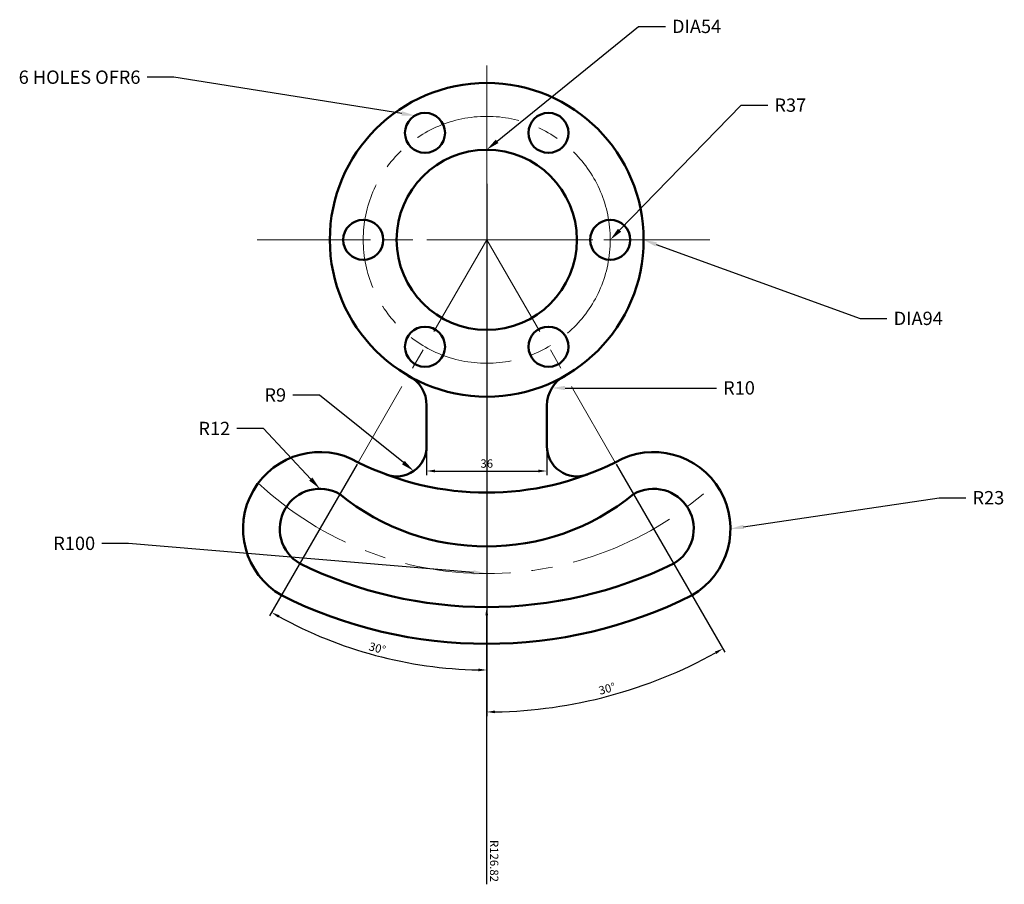
# Model space of a CAD drawing. Units: millimetres. Extents: x 2573 to 2868, y 2132 to 2391.
import ezdxf
from ezdxf import colors
from ezdxf.entities.mleader import LeaderData, LeaderLine
from ezdxf.math import Vec2, Vec3

# ---------------------------------------------------------------- set-up
doc = ezdxf.new("R2010")
doc.units = ezdxf.units.MM
doc.linetypes.add('CENTER', pattern=[50.8, 31.75, -6.35, 6.35, -6.35])
for name, color, linetype, lineweight in [('M-CNTR', 4, 'CENTER', 18), ('M-DIMS', 2, 'Continuous', 25), ('M-OUTL', 7, 'Continuous', 50)]:
    doc.layers.add(name, color=color, linetype=linetype, lineweight=lineweight)
doc.styles.get("Standard").update_dxf_attribs({"font": 'arial.ttf'})
doc.dimstyles.new('ISO-25', dxfattribs={"dimtxt": 2.5, "dimasz": 2.5, "dimexe": 1.25, "dimexo": 0.625, "dimtad": 1, "dimtxsty": 'Standard', "dimcen": 2.5, "dimadec": 0, "dimazin": 0, "dimtfac": 1, "dimtmove": 0, "dimatfit": 3, "dimfxl": 1, "dimarcsym": 0})

# ---------------------------------------------------------------- blocks, each defined once
blk = doc.blocks.new('*U1')
blk.add_circle((0, 0), 6)
blk = doc.blocks.new('*U2')
at = {"layer": 'M-OUTL', "color": 0, "linetype": 'ByBlock', "lineweight": -2, "transparency": 16777216}
for p, rotation in [((2694.13, 2357.36), 300), ((2731.13, 2357.36), 239.9999999999999), ((2749.63, 2325.31), 180), ((2694.13, 2293.27), 59.99999999999999), ((2731.13, 2293.27), 119.9999999999999)]:
    blk.add_blockref('*U1', p, dxfattribs=dict(at, rotation=rotation))
blk.add_blockref('*U1', (2675.63, 2325.31), dxfattribs=at)
blk = doc.blocks.new('*D3')
at = {"layer": 'Defpoints', "color": 0, "transparency": 16777216}
for p in [(2712.63, 2377.57), (2712.63, 2325.31), (2674.13, 2258.63), (2712.63, 2225.31), (2668.55, 2204.19)]:
    blk.add_point(p, dxfattribs=at)
at = {"layer": 'M-DIMS', "color": 0, "lineweight": -2, "transparency": 16777216}
for p, q in [((2673.82, 2258.09), (2647.56, 2212.6)), ((2712.63, 2224.69), (2712.63, 2195.16))]:
    blk.add_line(p, q, dxfattribs=at)
blk.add_arc((2712.63, 2325.31), 128.9, 241.1112, 268.8888, dxfattribs=at)
at = {"layer": 'M-DIMS', "color": 0, "transparency": 16777216}
for points in [[(2650.15, 2212.09), (2650.56, 2212.81), (2648.18, 2213.68)], [(2710.14, 2196.85), (2710.13, 2196.02), (2712.63, 2196.41)]]:
    blk.add_solid(points, dxfattribs=at)
at = {"layer": 'M-DIMS', "color": 0, "transparency": 16777216, "insert": (2679.76, 2202.64), "char_height": 2.5, "attachment_point": 5, "rotation": 345}
blk.add_mtext('30°', dxfattribs=at)
blk = doc.blocks.new('*D4')
at = {"layer": 'Defpoints', "color": 0, "transparency": 16777216}
for p in [(2712.63, 2377.57), (2712.63, 2325.31), (2751.13, 2258.63), (2712.63, 2225.31), (2737.2, 2185.99)]:
    blk.add_point(p, dxfattribs=at)
at = {"layer": 'M-DIMS', "color": 0, "lineweight": -2, "transparency": 16777216}
for p, q in [((2751.45, 2258.09), (2784, 2201.71)), ((2712.63, 2224.69), (2712.63, 2182.59))]:
    blk.add_line(p, q, dxfattribs=at)
blk.add_arc((2712.63, 2325.31), 141.47, 271.0125, 298.9875, dxfattribs=at)
at = {"layer": 'M-DIMS', "color": 0, "transparency": 16777216}
for points in [[(2780.99, 2201.93), (2781.4, 2201.2), (2783.37, 2202.8)], [(2715.14, 2183.45), (2715.13, 2184.28), (2712.63, 2183.84)]]:
    blk.add_solid(points, dxfattribs=at)
at = {"layer": 'M-DIMS', "color": 0, "transparency": 16777216, "insert": (2748.76, 2190.5), "char_height": 2.5, "attachment_point": 5, "rotation": 15}
blk.add_mtext('30°', dxfattribs=at)
blk = doc.blocks.new('*D5')
at = {"layer": 'Defpoints', "color": 0, "transparency": 16777216}
for p in [(2694.63, 2269.55), (2730.63, 2269.72), (2730.63, 2256.04)]:
    blk.add_point(p, dxfattribs=at)
at = {"layer": 'M-DIMS', "color": 0, "lineweight": -2, "transparency": 16777216}
for p, q in [((2694.63, 2268.93), (2694.63, 2254.79)), ((2730.63, 2269.09), (2730.63, 2254.79)), ((2697.13, 2256.04), (2728.13, 2256.04))]:
    blk.add_line(p, q, dxfattribs=at)
at = {"layer": 'M-DIMS', "color": 0, "transparency": 16777216}
for points in [[(2697.13, 2256.46), (2697.13, 2255.63), (2694.63, 2256.04)], [(2728.13, 2256.46), (2728.13, 2255.63), (2730.63, 2256.04)]]:
    blk.add_solid(points, dxfattribs=at)
at = {"layer": 'M-DIMS', "color": 0, "transparency": 16777216, "insert": (2712.63, 2257.95), "char_height": 2.5, "attachment_point": 5}
blk.add_mtext('36', dxfattribs=at)
blk = doc.blocks.new('*D6')
at = {"layer": 'Defpoints', "color": 0, "transparency": 16777216}
for p in [(2712.63, 2342.11), (2712.63, 2215.29)]:
    blk.add_point(p, dxfattribs=at)
at = {"layer": 'M-DIMS', "color": 0, "lineweight": -2, "transparency": 16777216}
for p, q in [((2712.63, 2342.11), (2712.63, 2215.29)), ((2712.63, 2132.19), (2712.63, 2212.79))]:
    blk.add_line(p, q, dxfattribs=at)
at = {"layer": 'M-DIMS', "color": 0, "transparency": 16777216}
blk.add_solid([(2713.05, 2212.79), (2712.22, 2212.79), (2712.63, 2215.29)], dxfattribs=at)
at = {"layer": 'M-DIMS', "color": 0, "transparency": 16777216, "insert": (2714.54, 2139.19), "char_height": 2.5, "attachment_point": 5, "rotation": 270.0002}
blk.add_mtext('R126.82', dxfattribs=at)

msp = doc.modelspace()

# ---------------------------------------------------------------- linework, layer by layer
at = {"layer": 'M-CNTR'}
for p, q in [((2712.634, 2325.315), (2712.634, 2377.572)), ((2712.634, 2377.572), (2712.634, 2225.315)), ((2779.418, 2325.315), (2643.865, 2325.315)), ((2643.865, 2325.315), (2712.634, 2325.315)), ((2712.634, 2325.315), (2674.134, 2258.631)), ((2712.634, 2325.315), (2779.418, 2325.315)), ((2712.634, 2325.315), (2751.134, 2258.631)), ((2668.634, 2249.104), (2651.134, 2218.793)), ((2756.634, 2249.104), (2774.134, 2218.793))]:
    msp.add_line(p, q, dxfattribs=at)
msp.add_circle((2712.634, 2325.315), 37, dxfattribs=at)
msp.add_arc((2712.634, 2325.315), 100, 226.79275, 313.20725, dxfattribs=at)
at = {"layer": 'M-OUTL'}
for p, q in [((2694.634, 2263.437), (2694.634, 2275.666)), ((2730.634, 2263.437), (2730.634, 2276.002))]:
    msp.add_line(p, q, dxfattribs=at)
for radius in [47, 27]:
    msp.add_circle((2712.634, 2325.315), radius, dxfattribs=at)
for centre, radius, start, end in [((2684.634, 2275.666), 10, 0, 63.30018), ((2740.634, 2275.666), 10, 116.69982, 180), ((2685.634, 2263.437), 9, 249.56325, 0), ((2739.634, 2263.437), 9, 180, 290.43675), ((2662.634, 2238.712), 23, 60, 240), ((2762.634, 2238.712), 23, 300, 120), ((2712.634, 2335.895), 86.326, 243.51354, 296.48646), ((2662.634, 2238.712), 12, 60, 240), ((2762.634, 2238.712), 12, 300, 120), ((2712.634, 2303.052), 69.616, 230.79916, 309.20084), ((2712.634, 2342.109), 126.823, 243.79653, 296.20347), ((2712.634, 2341.537), 137.289, 243.38703, 296.61297)]:
    msp.add_arc(centre, radius, start, end, dxfattribs=at)

# ---------------------------------------------------------------- block references
msp.add_blockref('*U2', (0, 0), dxfattribs=at)

# ---------------------------------------------------------------- dimensions: what is measured, and where the dimension line sits
at = {"layer": 'M-DIMS'}
for base, line1, line2, picture, middle in [((2668.546, 2204.185), ((2712.634, 2377.572), (2712.634, 2225.315)), ((2712.634, 2325.315), (2674.134, 2258.631)), '*D3', (2679.763, 2202.641)), ((2737.2, 2185.991), ((2712.634, 2325.315), (2751.134, 2258.631)), ((2712.634, 2377.572), (2712.634, 2225.315)), '*D4', (2748.757, 2190.5))]:
    dim = msp.add_angular_dim_2l(base=base, line1=line1, line2=line2, dimstyle='ISO-25', override={"dimclrd": 0, "dimclre": 0, "dimclrt": 0}, dxfattribs=at)
    dim.commit()
    dim.dimension.update_dxf_attribs({"geometry": picture, "text_midpoint": middle})
dim = msp.add_radius_dim(center=(2712.634, 2342.109), mpoint=(2712.634, 2215.286), dimstyle='ISO-25', override={"dimdec": 2, "dimlfac": 1, "dimrnd": 0, "dimzin": 0, "dimdsep": 46, "dimlunit": 2}, dxfattribs=at)
dim.commit()
dim.dimension.update_dxf_attribs({"geometry": '*D6', "text_midpoint": (2712.634, 2139.193), "dimtype": 164})
dim = msp.add_linear_dim(base=(2730.634, 2256.045), p1=(2694.634, 2269.551), p2=(2730.634, 2269.72), dimstyle='ISO-25', override={"dimclrd": 0, "dimclre": 0, "dimclrt": 0}, dxfattribs=at)
dim.commit()
dim.dimension.update_dxf_attribs({"geometry": '*D5', "text_midpoint": (2712.634, 2257.947)})

# ---------------------------------------------------------------- leaders
ml = msp.add_multileader_mtext('Standard', dxfattribs=at)
ml.set_content('DIA54', color=256)
ml.set_leader_properties()
ml.build(insert=Vec2(0, 0))
ctx = ml.context
ctx.base_point, ctx.plane_origin = Vec3(2766.136, 2389.243), Vec3(2712.634, 2352.315)
notes = []
notes.append((ctx, [(0, (1, 1, 0), (2758.136, 2389.243), (1, 0), 8, [(0, [(2712.634, 2352.315)], 0, [])])]))
ctx.mtext.insert, ctx.mtext.flow_direction = Vec3(2768.136, 2391.277), 5
ml = msp.add_multileader_mtext('Standard', dxfattribs=at)
ml.set_content('6 HOLES OFR6', color=256)
ml.set_leader_properties()
ml.build(insert=Vec2(0, 0))
ctx = ml.context
ctx.base_point, ctx.plane_origin = Vec3(2567.301, 2374.016), Vec3(2691.134, 2362.554)
ctx.text_align_type = 2
notes.append((ctx, [(0, (1, 1, 0), (2618.894, 2374.016), (-1, 0), 8, [(0, [(2691.134, 2362.554)], 0, [])])]))
ctx.mtext.insert, ctx.mtext.alignment, ctx.mtext.flow_direction = Vec3(2608.894, 2376.05), 3, 5
ml = msp.add_multileader_mtext('Standard', dxfattribs=at)
ml.set_content('R37', color=256)
ml.set_leader_properties()
ml.build(insert=Vec2(0, 0))
ctx = ml.context
ctx.base_point, ctx.plane_origin = Vec3(2796.804, 2365.642), Vec3(2749.634, 2325.315)
notes.append((ctx, [(0, (1, 1, 0), (2788.804, 2365.642), (1, 0), 8, [(0, [(2749.634, 2325.315)], 0, [])])]))
ctx.mtext.insert, ctx.mtext.flow_direction = Vec3(2798.804, 2367.677), 5
ml = msp.add_multileader_mtext('Standard', dxfattribs=at)
ml.set_content('DIA94', color=256)
ml.set_leader_properties()
ml.build(insert=Vec2(0, 0))
ctx = ml.context
ctx.base_point, ctx.plane_origin = Vec3(2832.533, 2301.746), Vec3(2759.634, 2325.315)
notes.append((ctx, [(0, (1, 1, 0), (2824.533, 2301.746), (1, 0), 8, [(0, [(2759.634, 2325.315)], 0, [])])]))
ctx.mtext.insert, ctx.mtext.flow_direction = Vec3(2834.533, 2303.78), 5
ml = msp.add_multileader_mtext('Standard', dxfattribs=at)
ml.set_content('R10', color=256)
ml.set_leader_properties()
ml.build(insert=Vec2(0, 0))
ctx = ml.context
ctx.base_point, ctx.plane_origin = Vec3(2781.441, 2280.913), Vec3(2732.121, 2280.913)
notes.append((ctx, [(0, (1, 1, 0), (2773.441, 2280.913), (1, 0), 8, [(0, [(2732.121, 2280.913)], 0, [])])]))
ctx.mtext.insert, ctx.mtext.flow_direction = Vec3(2783.441, 2282.947), 5
ml = msp.add_multileader_mtext('Standard', dxfattribs=at)
ml.set_content('R9', color=256)
ml.set_leader_properties()
ml.build(insert=Vec2(0, 0))
ctx = ml.context
ctx.base_point, ctx.plane_origin = Vec3(2644.062, 2278.788), Vec3(2690.768, 2256.045)
ctx.text_align_type = 2
notes.append((ctx, [(0, (1, 1, 0), (2662.521, 2278.788), (-1, 0), 8, [(0, [(2690.768, 2256.045)], 0, [])])]))
ctx.mtext.insert, ctx.mtext.alignment, ctx.mtext.flow_direction = Vec3(2652.521, 2280.823), 3, 5
ml = msp.add_multileader_mtext('Standard', dxfattribs=at)
ml.set_content('R12', color=256)
ml.set_leader_properties()
ml.build(insert=Vec2(0, 0))
ctx = ml.context
ctx.base_point, ctx.plane_origin = Vec3(2624.25, 2268.783), Vec3(2662.634, 2250.712)
ctx.text_align_type = 2
notes.append((ctx, [(0, (1, 1, 0), (2645.767, 2268.783), (-1, 0), 8, [(0, [(2662.634, 2250.712)], 0, [])])]))
ctx.mtext.insert, ctx.mtext.alignment, ctx.mtext.flow_direction = Vec3(2635.767, 2270.783), 3, 5
ml = msp.add_multileader_mtext('Standard', dxfattribs=at)
ml.set_content('R23', color=256)
ml.set_leader_properties()
ml.build(insert=Vec2(0, 0))
ctx = ml.context
ctx.base_point, ctx.plane_origin = Vec3(2856.158, 2248.001), Vec3(2785.634, 2238.712)
notes.append((ctx, [(0, (1, 1, 0), (2848.158, 2248.001), (1, 0), 8, [(0, [(2785.634, 2238.712)], 0, [])])]))
ctx.mtext.insert, ctx.mtext.flow_direction = Vec3(2858.158, 2250.037), 5
ml = msp.add_multileader_mtext('Standard', dxfattribs=at)
ml.set_content('R100', color=256)
ml.set_leader_properties()
ml.build(insert=Vec2(0, 0))
ctx = ml.context
ctx.base_point, ctx.plane_origin = Vec3(2580.675, 2234.339), Vec3(2712.634, 2225.315)
ctx.text_align_type = 2
notes.append((ctx, [(0, (1, 1, 0), (2605.328, 2234.339), (-1, 0), 8, [(0, [(2712.634, 2225.315)], 0, [])])]))
ctx.mtext.insert, ctx.mtext.alignment, ctx.mtext.flow_direction = Vec3(2595.328, 2236.373), 3, 5
for ctx, leaders in notes:
    for number, flags, end, landing, length, lines in leaders:
        leader = LeaderData()
        leader.index, (leader.has_last_leader_line, leader.has_dogleg_vector, leader.attachment_direction) = number, flags
        leader.last_leader_point, leader.dogleg_vector, leader.dogleg_length = Vec3(end), Vec3(landing), length
        for number, points, colour, breaks in lines:
            line = LeaderLine()
            line.index, line.vertices, line.color, line.breaks = number, Vec3.list(points), colors.encode_raw_color(colour), breaks
            leader.lines.append(line)
        ctx.leaders.append(leader)

doc.saveas('drawing.dxf')
